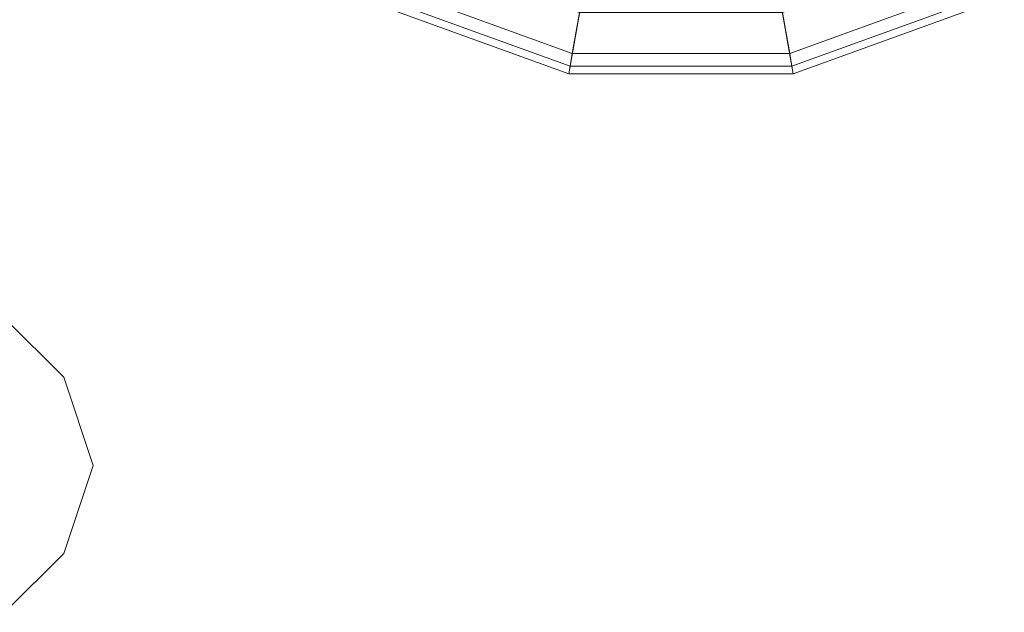
# Model space of a CAD drawing. Units: inches. Extents: x 375 to 1122, y 27 to 1069.
# Tile 40 of 155: x 717.878 to 719.94, y 296.625 to 297.867. Entities that reach past the tile are written whole.
import ezdxf

# ---------------------------------------------------------------- set-up
doc = ezdxf.new("R2010")
doc.units = ezdxf.units.IN
doc.layers.add('Furniture', color=30, linetype='Continuous', lineweight=18)

# ---------------------------------------------------------------- blocks, each defined once
blk = doc.blocks.new('A$C403C54AD')
for points in [[(1.2136, 0.863764, -0.031825), (1.180252, 0.857884, -0.028747), (1.180252, 0.857884, -0.028747), (1.209578, 0.874815, -0.031825)], [(1.210344, 0.86319, 0.131159), (1.213207, 0.863695, 0.117935), (1.209232, 0.874616, 0.117935), (1.206714, 0.873162, 0.131159)], [(1.210384, 0.863197, -0.028594), (1.2136, 0.863764, -0.031825), (1.209578, 0.874815, -0.031825), (1.206749, 0.873182, -0.028594)], [(1.213207, 0.863695, 0.117935), (1.212542, 0.863578, 0.089693), (1.208648, 0.874278, 0.089693), (1.209232, 0.874616, 0.117935)], [(1.212542, 0.863578, 0.089693), (1.207259, 0.862646, 0.071684), (1.204002, 0.871596, 0.071684), (1.208648, 0.874278, 0.089693)], [(1.2136, 0.852004, -0.031825), (1.180252, 0.857884, -0.028747), (1.180252, 0.857884, -0.028747), (1.2136, 0.863764, -0.031825)], [(1.210344, 0.852578, 0.131159), (1.213207, 0.852073, 0.117935), (1.213207, 0.863695, 0.117935), (1.210344, 0.86319, 0.131159)], [(1.210384, 0.852571, -0.028594), (1.2136, 0.852004, -0.031825), (1.2136, 0.863764, -0.031825), (1.210384, 0.863197, -0.028594)], [(1.213207, 0.852073, 0.117935), (1.212542, 0.85219, 0.089693), (1.212542, 0.863578, 0.089693), (1.213207, 0.863695, 0.117935)], [(1.212542, 0.85219, 0.089693), (1.207259, 0.853122, 0.071684), (1.207259, 0.862646, 0.071684), (1.212542, 0.863578, 0.089693)], [(1.209578, 0.840953, -0.031825), (1.180252, 0.857884, -0.028747), (1.180252, 0.857884, -0.028747), (1.2136, 0.852004, -0.031825)], [(1.208648, 0.84149, 0.089693), (1.204002, 0.844172, 0.071684), (1.207259, 0.853122, 0.071684), (1.212542, 0.85219, 0.089693)], [(1.206714, 0.842606, 0.131159), (1.209232, 0.841152, 0.117935), (1.213207, 0.852073, 0.117935), (1.210344, 0.852578, 0.131159)], [(1.206749, 0.842586, -0.028594), (1.209578, 0.840953, -0.031825), (1.2136, 0.852004, -0.031825), (1.210384, 0.852571, -0.028594)], [(1.209232, 0.841152, 0.117935), (1.208648, 0.84149, 0.089693), (1.212542, 0.85219, 0.089693), (1.213207, 0.852073, 0.117935)]]:
    blk.add_3dface(points)
for points, invisible_edges in [([(1.234124, 0.8271, -0.024899), (1.234124, 0.8271, -0.024899), (1.238741, 0.825561, -0.024899), (1.229506, 0.825561, -0.024899)], 4), ([(1.234124, 0.8271, -0.026438), (1.234124, 0.8271, -0.026438), (1.238741, 0.825561, -0.026438), (1.229506, 0.825561, -0.026438)], 4), ([(1.234124, 0.8271, -0.024899), (1.234124, 0.8271, -0.026438), (1.229506, 0.825561, -0.026438), (1.229506, 0.825561, -0.024899)], 4), ([(1.238741, 0.825561, -0.026438), (1.238741, 0.825561, -0.024899), (1.234124, 0.8271, -0.024899), (1.234124, 0.8271, -0.026438)], 1), ([(1.238741, 0.825561, -0.024899), (1.229506, 0.825561, -0.024899), (1.226428, 0.822483, -0.024899), (1.24182, 0.822483, -0.024899)], 5), ([(1.238741, 0.825561, -0.026438), (1.229506, 0.825561, -0.026438), (1.226428, 0.822483, -0.026438), (1.24182, 0.822483, -0.026438)], 5), ([(1.229506, 0.825561, -0.026438), (1.229506, 0.825561, -0.024899), (1.226428, 0.822483, -0.024899), (1.226428, 0.822483, -0.026438)], 5), ([(1.24182, 0.822483, -0.024899), (1.24182, 0.822483, -0.026438), (1.238741, 0.825561, -0.026438), (1.238741, 0.825561, -0.024899)], 5)]:
    blk.add_3dface(points, dxfattribs=dict(invisible_edges=invisible_edges))

msp = doc.modelspace()

# ---------------------------------------------------------------- block references
at = {"layer": 'Furniture', "xscale": 39.9918517141215, "yscale": 39.9918517141215, "zscale": 39.9918517141215, "rotation": 270}
msp.add_blockref('A$C403C54AD', (684.9549, 346.2875, 0.024), dxfattribs=at)

doc.saveas('drawing.dxf')
